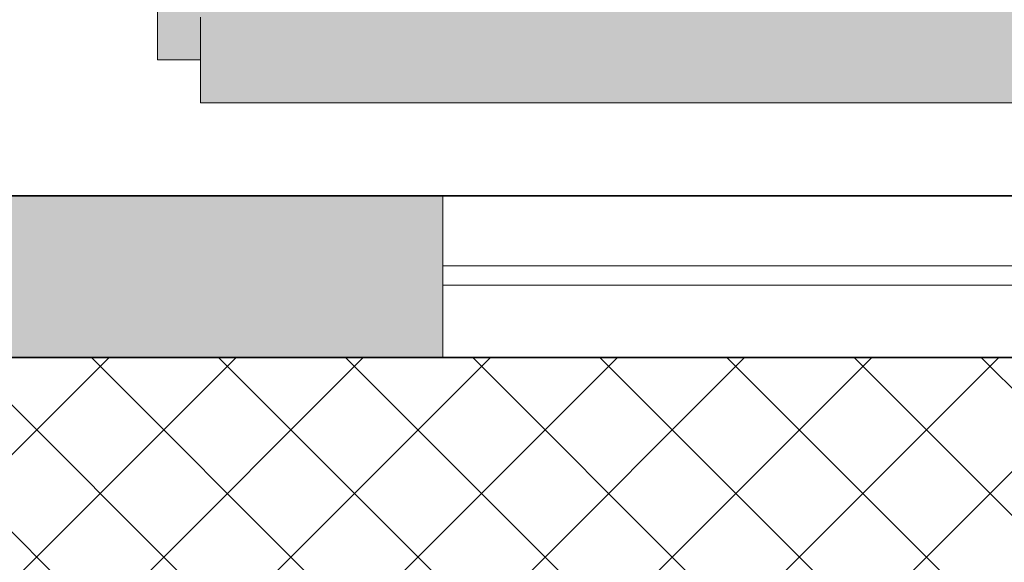
# Model space of a CAD drawing. Units: inches. Extents: x 2167 to 2589, y 1680 to 2489.
# Tile 23 of 38: x 2251 to 2306, y 1835 to 1865. Entities that reach past the tile are written whole.
import ezdxf

# ---------------------------------------------------------------- set-up
doc = ezdxf.new("R2010")
doc.units = ezdxf.units.IN
doc.header["$MEASUREMENT"] = 0
for name, color, linetype, lineweight in [('A-FURN-PATT', 31, 'Continuous', 13), ('A-WALL-PATT', 250, 'Continuous', 13), ('furniture', 34, 'Continuous', 18), ('L-PVMT-PATT', 252, 'Continuous', 13), ('walls', 7, 'Continuous', 35), ('windows', 141, 'Continuous', 18)]:
    doc.layers.add(name, color=color, linetype=linetype, lineweight=lineweight)

# ---------------------------------------------------------------- blocks, each defined once
blk = doc.blocks.new('FABRIC SOFA 4S')
at = {"layer": 'furniture'}
for p, q in [((3, 54), (34, 54)), ((3, 51), (3, 54)), ((0, -51), (0, 51)), ((6, 51), (0, 51))]:
    blk.add_line(p, q, dxfattribs=at)

msp = doc.modelspace()

# ---------------------------------------------------------------- hatches: boundary and pattern name
at = {"layer": 'A-FURN-PATT'}
h = msp.add_hatch(color=256, dxfattribs=at)
h.dxf.hatch_style = 1
h.paths.add_polyline_path([(2263.924, 1886.408), (2263.924, 1869.74), (2282.825, 1869.74), (2282.825, 1886.408)])
h.paths.add_polyline_path([(2282.825, 1886.408), (2282.825, 1869.74), (2301.725, 1869.74), (2301.725, 1886.408)])
h.paths.add_polyline_path([(2301.725, 1886.408), (2301.725, 1869.74), (2320.625, 1869.74), (2320.625, 1886.408)])
h.paths.add_polyline_path([(2320.625, 1886.408), (2320.625, 1869.74), (2339.525, 1869.74), (2339.525, 1886.408)])
h.paths.add_polyline_path([(2263.924, 1869.74), (2261.245, 1864.978), (2342.204, 1864.978), (2339.525, 1869.74)])
h.paths.add_polyline_path([(2261.245, 1864.978), (2261.245, 1860.216), (2342.204, 1860.216), (2342.204, 1864.978)])
h.paths.add_polyline_path([(2258.864, 1887.202), (2258.864, 1862.597), (2261.245, 1862.597), (2261.245, 1864.978), (2263.627, 1869.211), (2263.627, 1887.202)])
h.paths.add_polyline_path([(2339.823, 1887.202), (2339.823, 1869.211), (2342.204, 1864.978), (2342.204, 1862.597), (2344.585, 1862.597), (2344.585, 1887.202)])
at = {"layer": 'A-WALL-PATT'}
h = msp.add_hatch(color=256, dxfattribs=at)
h.dxf.hatch_style = 1
h.paths.add_polyline_path([(2274.738, 1855.042), (2224.048, 1855.042), (2224.048, 2003.119), (2215.048, 2003.119), (2215.048, 1846.042), (2274.738, 1846.042)])
h.paths.add_polyline_path([(2354.886, 1855.042), (2330.895, 1855.042), (2330.895, 1846.042), (2354.773, 1846.042), (2354.773, 1852.042, -0.01877)])
h.paths.add_polyline_path([(2422.048, 1864.695), (2426.208, 1864.695), (2426.208, 1867.924), (2426.208, 1869.195), (2422.048, 1869.195), (2422.048, 1916.243), (2417.548, 1916.243), (2417.548, 1855.042), (2394.773, 1855.042), (2394.773, 1852.042), (2394.773, 1846.042), (2417.548, 1846.042), (2417.548, 1779.195), (2427.738, 1779.195), (2427.738, 1783.941), (2427.738, 1788.195), (2422.048, 1788.195)])
at = {"layer": 'L-PVMT-PATT'}
h = msp.add_hatch(dxfattribs=at)
h.set_pattern_fill('ANSI37', color=256, scale=40)
h.paths.add_polyline_path([(2417.548, 1783.695), (2417.548, 1846.042), (2239.361, 1846.042), (2239.361, 1687.695), (2369.843, 1687.695), (2369.843, 1696.695), (2375.607, 1696.695), (2416.107, 1696.695), (2417.548, 1696.695)])

# ---------------------------------------------------------------- linework, layer by layer
at = {"layer": 'walls'}
for p, q in [((2224.048, 1855.042), (2354.886, 1855.042)), ((2215.048, 1846.042), (2417.548, 1846.042))]:
    msp.add_line(p, q, dxfattribs=at)
at = {"layer": 'windows'}
for p, q in [((2274.738, 1855.042), (2274.738, 1846.042)), ((2330.895, 1855.042), (2274.738, 1855.042)), ((2274.738, 1855.042), (2274.738, 1851.135)), ((2274.738, 1851.135), (2330.895, 1851.135)), ((2330.895, 1850.068), (2274.738, 1850.068)), ((2274.738, 1846.042), (2330.895, 1846.042))]:
    msp.add_line(p, q, dxfattribs=at)

# ---------------------------------------------------------------- block references
at = {"layer": 'furniture', "xscale": 0.7937147270336093, "yscale": 0.7937147270336093, "zscale": 0.7937147270336093, "rotation": 90}
msp.add_blockref('FABRIC SOFA 4S', (2301.725, 1860.216), dxfattribs=at)

doc.saveas('drawing.dxf')
